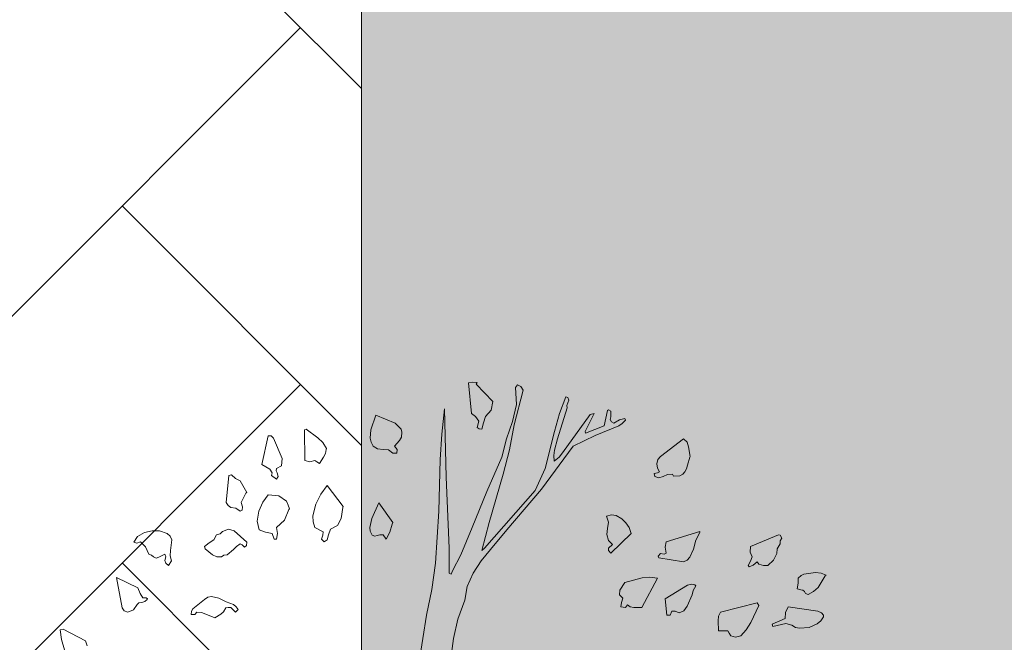
# Model space of a CAD drawing. Units: inches. Extents: x 84 to 1044, y -280 to 906.
# Tile 5 of 105: x 441 to 481, y -104 to -79. Entities that reach past the tile are written whole.
import ezdxf

# ---------------------------------------------------------------- set-up
doc = ezdxf.new("R2010")
doc.units = ezdxf.units.IN
doc.layers.add('L-HRDS', color=32, linetype='Continuous', lineweight=18)
doc.layers.add('L-PLNT', color=114, linetype='Continuous', lineweight=15)
doc.layers.add('L-PLNT-PATT', color=9, linetype='Continuous', lineweight=9, true_color=0xafd9aa)
doc.layers.add('L-PRKG-PATT', color=35, linetype='Continuous', lineweight=9, true_color=0x947764)

# ---------------------------------------------------------------- blocks, each defined once
blk = doc.blocks.new('A$C37E508DF')
for p, q in [((0.6329, 1.5111), (0.6367, 1.5175)), ((0.6367, 1.5175), (0.6423, 1.5201)), ((0.6423, 1.5201), (0.6453, 1.5158)), ((0.6453, 1.5158), (0.644, 1.4879)), ((0.6826, 1.493), (0.7096, 1.5209)), ((0.7083, 1.5239), (0.7152, 1.5244)), ((0.7096, 1.5209), (0.7083, 1.5239)), ((0.7152, 1.5244), (0.7225, 1.5231)), ((0.7225, 1.5231), (0.7174, 1.4729)), ((0.5583, 1.4948), (0.5596, 1.4995)), ((0.5596, 1.4995), (0.563, 1.5003)), ((0.563, 1.5003), (0.5737, 1.4733)), ((0.6475, 1.4545), (0.6329, 1.5111)), ((0.5596, 1.4905), (0.5583, 1.4948)), ((0.5613, 1.4862), (0.5596, 1.4905)), ((0.5608, 1.4823), (0.5613, 1.4862)), ((0.5767, 1.4317), (0.5608, 1.4823)), ((0.644, 1.4879), (0.6505, 1.46)), ((0.6852, 1.4785), (0.6826, 1.493)), ((0.7589, 1.3691), (0.7615, 1.481)), ((0.7615, 1.481), (0.7658, 1.4395)), ((0.4657, 1.4622), (0.4669, 1.4652)), ((0.4669, 1.4652), (0.4755, 1.463)), ((0.4897, 1.4772), (0.4935, 1.4789)), ((0.4897, 1.4678), (0.4897, 1.4772)), ((0.4905, 1.4635), (0.4897, 1.4678)), ((0.4935, 1.4789), (0.4952, 1.478)), ((0.4952, 1.478), (0.5004, 1.4532)), ((0.5313, 1.4437), (0.5167, 1.4729)), ((0.5167, 1.4729), (0.5231, 1.4716)), ((0.5231, 1.4716), (0.5686, 1.409)), ((0.5737, 1.4733), (0.5814, 1.4437)), ((0.6946, 1.4682), (0.6852, 1.4785)), ((0.6976, 1.4579), (0.6946, 1.4682)), ((0.7109, 1.4682), (0.7053, 1.4609)), ((0.7174, 1.4729), (0.7109, 1.4682)), ((0.8421, 1.4575), (0.8739, 1.4703)), ((0.8739, 1.4703), (0.882, 1.4463)), ((0.4708, 1.4566), (0.4657, 1.4622)), ((0.4764, 1.4532), (0.4708, 1.4566)), ((0.4755, 1.463), (0.4845, 1.4575)), ((0.5154, 1.4373), (0.4764, 1.4532)), ((0.4845, 1.4575), (0.4884, 1.4596)), ((0.4884, 1.4596), (0.4905, 1.4635)), ((0.5004, 1.4532), (0.5308, 1.4412)), ((0.6552, 1.4137), (0.6475, 1.4545)), ((0.6505, 1.46), (0.6603, 1.4317)), ((0.7002, 1.4476), (0.6976, 1.4579)), ((0.7083, 1.4502), (0.7049, 1.448)), ((0.7053, 1.4609), (0.7083, 1.4502)), ((0.8323, 1.4476), (0.8357, 1.451)), ((0.8357, 1.451), (0.8421, 1.4575)), ((0.551, 1.4197), (0.5154, 1.4373)), ((0.5308, 1.4412), (0.5313, 1.4437)), ((0.5814, 1.4437), (0.5969, 1.3833)), ((0.7049, 1.448), (0.7002, 1.4476)), ((0.7658, 1.4395), (0.7684, 1.3979)), ((0.831, 1.4424), (0.8323, 1.4476)), ((0.8318, 1.4343), (0.831, 1.4424)), ((0.8353, 1.4292), (0.8318, 1.4343)), ((0.8829, 1.433), (0.8816, 1.4262)), ((0.882, 1.4463), (0.8829, 1.433)), ((0.9605, 1.4257), (0.9686, 1.4334)), ((0.9686, 1.4334), (0.9875, 1.4476)), ((0.9875, 1.4476), (0.9905, 1.4467)), ((0.9905, 1.4467), (0.9896, 1.3966)), ((1.0269, 1.3996), (1.0411, 1.433)), ((1.0411, 1.433), (1.045, 1.4365)), ((1.045, 1.4365), (1.0497, 1.4369)), ((1.0497, 1.4369), (1.0604, 1.3901)), ((0.3598, 1.403), (0.3628, 1.4189)), ((0.3628, 1.4189), (0.3649, 1.4266)), ((0.3649, 1.4266), (0.3709, 1.4317)), ((0.3709, 1.4317), (0.4086, 1.403)), ((0.6029, 1.3494), (0.551, 1.4197)), ((0.5814, 1.4133), (0.5767, 1.4317)), ((0.6603, 1.4317), (0.668, 1.4021)), ((0.8434, 1.4197), (0.8353, 1.4292)), ((0.8391, 1.4141), (0.8434, 1.4197)), ((0.8781, 1.4197), (0.8709, 1.4154)), ((0.8816, 1.4262), (0.8781, 1.4197)), ((0.9545, 1.4159), (0.9605, 1.4257)), ((0.3602, 1.4021), (0.3598, 1.403)), ((0.364, 1.3888), (0.3602, 1.4021)), ((0.4086, 1.403), (0.4125, 1.3979)), ((0.5686, 1.409), (0.5741, 1.4021)), ((0.5741, 1.4021), (0.5823, 1.3953)), ((0.5827, 1.4043), (0.5814, 1.4133)), ((0.5823, 1.3953), (0.5827, 1.4043)), ((0.6655, 1.3743), (0.6552, 1.4137)), ((0.668, 1.4021), (0.6925, 1.3455)), ((0.8395, 1.4086), (0.8391, 1.4141)), ((0.846, 1.4086), (0.8395, 1.4086)), ((0.8528, 1.4137), (0.846, 1.4086)), ((0.8619, 1.4146), (0.8528, 1.4137)), ((0.8709, 1.4154), (0.8619, 1.4146)), ((0.9549, 1.4146), (0.9545, 1.4159)), ((0.9558, 1.4077), (0.9549, 1.4146)), ((0.9592, 1.4017), (0.9558, 1.4077)), ((0.966, 1.3914), (0.9592, 1.4017)), ((0.3657, 1.3828), (0.364, 1.3888)), ((0.4125, 1.3979), (0.4142, 1.391)), ((0.4142, 1.391), (0.4134, 1.3837)), ((0.7684, 1.3979), (0.771, 1.3134)), ((0.9703, 1.3944), (0.966, 1.3914)), ((0.9733, 1.3966), (0.9703, 1.3944)), ((0.9819, 1.3944), (0.9733, 1.3966)), ((0.9896, 1.3966), (0.9819, 1.3944)), ((1.0282, 1.3876), (1.0269, 1.3996)), ((1.0359, 1.3833), (1.0282, 1.3876)), ((1.0604, 1.3901), (1.0471, 1.3824)), ((0.3683, 1.3781), (0.3657, 1.3828)), ((0.3718, 1.3738), (0.3683, 1.3781)), ((0.3765, 1.3713), (0.3718, 1.3738)), ((0.3872, 1.3708), (0.3765, 1.3713)), ((0.3885, 1.3738), (0.3872, 1.3708)), ((0.3971, 1.3734), (0.3885, 1.3738)), ((0.4039, 1.3704), (0.3971, 1.3734)), ((0.4108, 1.3683), (0.4039, 1.3704)), ((0.4134, 1.3837), (0.4099, 1.3781)), ((0.4099, 1.3781), (0.4134, 1.376)), ((0.4176, 1.37), (0.4108, 1.3683)), ((0.4134, 1.376), (0.4189, 1.3751)), ((0.4189, 1.3751), (0.4176, 1.37)), ((0.5969, 1.3833), (0.6132, 1.3472)), ((0.6882, 1.2949), (0.6655, 1.3743)), ((0.7538, 1.2529), (0.7589, 1.3691)), ((1.0334, 1.37), (1.0351, 1.376)), ((1.0359, 1.3661), (1.0334, 1.37)), ((1.0351, 1.376), (1.0368, 1.3794)), ((1.0368, 1.3794), (1.0359, 1.3833)), ((1.0441, 1.3717), (1.0359, 1.3661)), ((1.0471, 1.3824), (1.0432, 1.3764)), ((1.0432, 1.3764), (1.0441, 1.3717)), ((1.1033, 1.367), (1.1097, 1.373)), ((1.1097, 1.373), (1.114, 1.3717)), ((1.114, 1.3717), (1.1183, 1.328)), ((0.9274, 1.3215), (0.9532, 1.3554)), ((0.9532, 1.3554), (0.9635, 1.3413)), ((1.0848, 1.3443), (1.0955, 1.3631)), ((1.0955, 1.3631), (1.1033, 1.367)), ((0.6595, 1.2829), (0.6029, 1.3494)), ((0.6132, 1.3472), (0.6959, 1.2529)), ((0.6925, 1.3455), (0.7161, 1.2868)), ((0.9635, 1.3413), (0.9721, 1.325)), ((1.0197, 1.3297), (1.0321, 1.3387)), ((1.0321, 1.3387), (1.0497, 1.3404)), ((1.0497, 1.3404), (1.0587, 1.3284)), ((1.0861, 1.343), (1.0848, 1.3443)), ((1.0938, 1.328), (1.0861, 1.343)), ((0.846, 1.2949), (0.8687, 1.3271)), ((0.8687, 1.3271), (0.8803, 1.3014)), ((0.9279, 1.3194), (0.9274, 1.3215)), ((0.9721, 1.325), (0.9768, 1.3061)), ((1.0149, 1.3172), (1.0171, 1.3232)), ((1.0171, 1.3232), (1.0197, 1.3297)), ((1.0587, 1.3284), (1.0651, 1.3134)), ((1.0917, 1.3207), (1.0938, 1.328)), ((1.0925, 1.3151), (1.0917, 1.3207)), ((1.1153, 1.3228), (1.111, 1.3194)), ((1.1183, 1.328), (1.1153, 1.3228)), ((0.4717, 1.3009), (0.4807, 1.3065)), ((0.4807, 1.3065), (0.4884, 1.3074)), ((0.4884, 1.3074), (0.4965, 1.3057)), ((0.4965, 1.3057), (0.4935, 1.2954)), ((0.771, 1.3134), (0.7761, 1.2285)), ((0.9305, 1.3018), (0.9279, 1.3194)), ((0.9768, 1.3061), (0.9763, 1.2962)), ((1.0162, 1.3164), (1.0149, 1.3172)), ((1.0231, 1.2988), (1.0162, 1.3164)), ((1.0651, 1.3134), (1.0677, 1.2975)), ((1.0955, 1.3138), (1.0925, 1.3151)), ((1.1028, 1.3185), (1.0955, 1.3138)), ((1.111, 1.3194), (1.1028, 1.3185)), ((0.4597, 1.2868), (0.4648, 1.2945)), ((0.4648, 1.2945), (0.4717, 1.3009)), ((0.4935, 1.2954), (0.4948, 1.2855)), ((0.7002, 1.2495), (0.6882, 1.2949)), ((0.8473, 1.2924), (0.846, 1.2949)), ((0.8507, 1.2795), (0.8473, 1.2924)), ((0.8803, 1.3014), (0.8833, 1.2872)), ((0.9365, 1.2902), (0.9305, 1.3018)), ((0.9476, 1.2842), (0.9365, 1.2902)), ((0.9763, 1.2962), (0.9733, 1.2868)), ((1.0359, 1.2868), (1.0231, 1.2988)), ((1.0677, 1.2975), (1.0647, 1.2829)), ((0.2101, 1.2696), (0.2127, 1.2744)), ((0.2127, 1.2744), (0.2152, 1.2752)), ((0.2152, 1.2752), (0.2611, 1.2559)), ((0.3439, 1.2804), (0.3992, 1.2636)), ((0.3439, 1.2787), (0.3439, 1.2804)), ((0.3507, 1.2662), (0.3439, 1.2787)), ((0.4562, 1.2774), (0.4597, 1.2868)), ((0.4897, 1.2452), (0.4562, 1.2774)), ((0.4961, 1.2756), (0.4935, 1.2658)), ((0.4948, 1.2855), (0.4961, 1.2756)), ((0.6865, 1.2508), (0.6595, 1.2829)), ((0.7161, 1.2868), (0.7349, 1.2422)), ((0.8567, 1.2679), (0.8507, 1.2795)), ((0.8619, 1.2752), (0.8567, 1.2679)), ((0.867, 1.2752), (0.8619, 1.2752)), ((0.8713, 1.2739), (0.867, 1.2752)), ((0.8756, 1.2726), (0.8713, 1.2739)), ((0.8799, 1.2744), (0.8756, 1.2726)), ((0.8829, 1.2808), (0.8799, 1.2744)), ((0.8833, 1.2872), (0.8829, 1.2808)), ((0.951, 1.2748), (0.9476, 1.2842)), ((0.9532, 1.2666), (0.951, 1.2748)), ((0.9733, 1.2868), (0.9596, 1.2799)), ((0.9596, 1.2799), (0.9605, 1.2744)), ((0.9605, 1.2744), (0.9626, 1.2679)), ((1.0347, 1.2769), (1.0359, 1.2868)), ((1.0359, 1.2679), (1.0347, 1.2769)), ((1.0432, 1.2774), (1.0402, 1.2679)), ((1.0544, 1.2791), (1.0432, 1.2774)), ((1.0647, 1.2829), (1.0544, 1.2791)), ((1.0848, 1.2628), (1.1054, 1.2817)), ((1.1054, 1.2817), (1.1148, 1.2842)), ((1.1148, 1.2842), (1.1247, 1.2804)), ((1.1247, 1.2804), (1.1281, 1.2765)), ((1.1281, 1.2765), (1.1341, 1.2752)), ((1.1341, 1.2752), (1.1384, 1.2666)), ((1.2075, 1.2666), (1.21, 1.2726)), ((1.21, 1.2726), (1.2147, 1.2774)), ((1.2147, 1.2774), (1.2276, 1.2817)), ((1.2276, 1.2817), (1.2392, 1.2817)), ((1.2392, 1.2817), (1.2521, 1.2787)), ((1.2521, 1.2787), (1.2632, 1.2722)), ((1.2632, 1.2722), (1.2692, 1.2628)), ((0.2127, 1.2654), (0.2101, 1.2696)), ((0.2127, 1.2602), (0.2127, 1.2654)), ((0.2174, 1.2521), (0.2127, 1.2602)), ((0.2611, 1.2559), (0.262, 1.2465)), ((0.3546, 1.2516), (0.3507, 1.2662)), ((0.3992, 1.2636), (0.4005, 1.2546)), ((0.4935, 1.2658), (0.4867, 1.2589)), ((0.4867, 1.2589), (0.4935, 1.2529)), ((0.9583, 1.2636), (0.9532, 1.2666)), ((0.9626, 1.2679), (0.9583, 1.2636)), ((1.0402, 1.2679), (1.0359, 1.2679)), ((1.0852, 1.2576), (1.0848, 1.2628)), ((1.0883, 1.2546), (1.0852, 1.2576)), ((1.0921, 1.2585), (1.0883, 1.2546)), ((1.0955, 1.2602), (1.0921, 1.2585)), ((1.1015, 1.2559), (1.0955, 1.2602)), ((1.1063, 1.2508), (1.1015, 1.2559)), ((1.1384, 1.2666), (1.1461, 1.2619)), ((1.1461, 1.2619), (1.1539, 1.2559)), ((1.1539, 1.2559), (1.1526, 1.2521)), ((1.2096, 1.2491), (1.2075, 1.2666)), ((1.2585, 1.2636), (1.2503, 1.2551)), ((1.2645, 1.2615), (1.2585, 1.2636)), ((1.2692, 1.2628), (1.2645, 1.2615)), ((0.2182, 1.2443), (0.2174, 1.2521)), ((0.2234, 1.2336), (0.2182, 1.2443)), ((0.262, 1.2465), (0.2586, 1.2388)), ((0.3602, 1.2383), (0.3546, 1.2516)), ((0.4005, 1.2546), (0.3992, 1.2452)), ((0.3992, 1.2452), (0.4026, 1.2431)), ((0.4026, 1.2431), (0.4086, 1.2443)), ((0.4086, 1.2443), (0.4121, 1.2401)), ((0.4121, 1.2401), (0.4112, 1.2375)), ((0.4931, 1.2491), (0.4897, 1.2452)), ((0.4935, 1.2529), (0.4931, 1.2491)), ((0.7015, 1.2323), (0.6865, 1.2508)), ((0.6959, 1.2529), (0.7002, 1.2495)), ((0.7349, 1.2422), (0.7482, 1.216)), ((0.7538, 1.2122), (0.7538, 1.2529)), ((1.117, 1.2422), (1.1063, 1.2508)), ((1.1221, 1.2418), (1.117, 1.2422)), ((1.126, 1.2388), (1.1221, 1.2418)), ((1.141, 1.2422), (1.1337, 1.2388)), ((1.1526, 1.2521), (1.141, 1.2422)), ((1.2079, 1.2323), (1.21, 1.2409)), ((1.21, 1.2409), (1.2096, 1.2491)), ((1.2186, 1.2431), (1.2173, 1.2392)), ((1.2285, 1.2383), (1.2186, 1.2431)), ((1.2405, 1.2418), (1.2371, 1.2388)), ((1.2448, 1.2431), (1.2405, 1.2418)), ((1.2503, 1.2551), (1.2448, 1.2431)), ((0.2328, 1.2251), (0.2234, 1.2336)), ((0.2401, 1.2251), (0.2328, 1.2251)), ((0.2474, 1.2268), (0.2401, 1.2251)), ((0.2504, 1.2306), (0.2474, 1.2268)), ((0.2568, 1.2255), (0.2504, 1.2306)), ((0.2633, 1.2229), (0.2568, 1.2255)), ((0.2586, 1.2388), (0.2611, 1.2319)), ((0.2611, 1.2319), (0.265, 1.2251)), ((0.265, 1.2251), (0.2633, 1.2229)), ((0.3649, 1.2336), (0.3602, 1.2383)), ((0.3709, 1.2306), (0.3649, 1.2336)), ((0.4112, 1.2375), (0.3709, 1.2306)), ((0.7148, 1.2126), (0.7015, 1.2323)), ((0.7761, 1.2285), (0.7821, 1.1856)), ((1.1337, 1.2388), (1.126, 1.2388)), ((1.2126, 1.2251), (1.2079, 1.2323)), ((1.2169, 1.2285), (1.2126, 1.2251)), ((1.2186, 1.2332), (1.2169, 1.2285)), ((1.2173, 1.2392), (1.2186, 1.2332)), ((1.2328, 1.2366), (1.2285, 1.2383)), ((1.2371, 1.2388), (1.2328, 1.2366)), ((0.1376, 1.2092), (0.1458, 1.2126)), ((0.1389, 1.2079), (0.1376, 1.2092)), ((0.1505, 1.189), (0.1389, 1.2079)), ((0.1458, 1.2126), (0.1548, 1.2135)), ((0.1548, 1.2135), (0.1741, 1.2109)), ((0.1741, 1.2109), (0.1784, 1.2083)), ((0.1784, 1.2083), (0.1831, 1.204)), ((0.7246, 1.1908), (0.7148, 1.2126)), ((0.7482, 1.216), (0.7508, 1.2109)), ((0.7508, 1.2109), (0.7538, 1.2122)), ((0.1831, 1.204), (0.1831, 1.1959)), ((0.1831, 1.1959), (0.1848, 1.1865)), ((0.3507, 1.1916), (0.352, 1.1933)), ((0.355, 1.1839), (0.3507, 1.1916)), ((0.352, 1.1933), (0.3576, 1.1942)), ((0.3576, 1.1942), (0.364, 1.1929)), ((0.364, 1.1929), (0.4005, 1.1702)), ((0.4134, 1.204), (0.4258, 1.2058)), ((0.4391, 1.156), (0.4134, 1.204)), ((0.4258, 1.2058), (0.4382, 1.2045)), ((0.4382, 1.2045), (0.4669, 1.1972)), ((0.4669, 1.1972), (0.4747, 1.1843)), ((1.2628, 1.1882), (1.2975, 1.2053)), ((1.2975, 1.2053), (1.2885, 1.1556)), ((0.1582, 1.1822), (0.1505, 1.189)), ((0.1668, 1.1775), (0.1582, 1.1822)), ((0.1711, 1.1792), (0.1668, 1.1775)), ((0.1728, 1.1826), (0.1711, 1.1792)), ((0.1758, 1.1847), (0.1728, 1.1826)), ((0.1788, 1.1852), (0.1758, 1.1847)), ((0.1848, 1.1865), (0.1788, 1.1852)), ((0.3563, 1.177), (0.355, 1.1839)), ((0.3645, 1.1586), (0.3563, 1.177)), ((0.4751, 1.177), (0.47, 1.1714)), ((0.4747, 1.1843), (0.4751, 1.177)), ((0.7281, 1.168), (0.7246, 1.1908)), ((0.7821, 1.1856), (0.7911, 1.1436)), ((1.2546, 1.1719), (1.2589, 1.1792)), ((1.2589, 1.1792), (1.2628, 1.1882)), ((0.2478, 1.1594), (0.2504, 1.1637)), ((0.2607, 1.1316), (0.2478, 1.1594)), ((0.2504, 1.1637), (0.3104, 1.1487)), ((0.4005, 1.1702), (0.3979, 1.1436)), ((0.4622, 1.1607), (0.458, 1.1573)), ((0.4657, 1.156), (0.4622, 1.1607)), ((0.47, 1.1714), (0.4721, 1.1646)), ((0.4721, 1.1646), (0.473, 1.1573)), ((0.7396, 1.1371), (0.7281, 1.168)), ((1.102, 1.1573), (1.1063, 1.1612)), ((1.1063, 1.1612), (1.1187, 1.1655)), ((1.1187, 1.1655), (1.1307, 1.1714)), ((1.1307, 1.1714), (1.1423, 1.1744)), ((1.1423, 1.1744), (1.1483, 1.1732)), ((1.1483, 1.1732), (1.1539, 1.1693)), ((1.1539, 1.1693), (1.1727, 1.1543)), ((1.2469, 1.1702), (1.2495, 1.1723)), ((1.2478, 1.1693), (1.2469, 1.1702)), ((1.2516, 1.1659), (1.2478, 1.1693)), ((1.2495, 1.1723), (1.2546, 1.1719)), ((1.2563, 1.1646), (1.2516, 1.1659)), ((1.2611, 1.1637), (1.2563, 1.1646)), ((1.2641, 1.1612), (1.2611, 1.1637)), ((1.2701, 1.1522), (1.2641, 1.1612)), ((0.1419, 1.1436), (0.1449, 1.1474)), ((0.1419, 1.141), (0.1419, 1.1436)), ((0.1449, 1.1474), (0.1509, 1.1504)), ((0.1509, 1.1504), (0.1994, 1.1573)), ((0.1994, 1.1573), (0.2041, 1.1479)), ((0.2041, 1.1479), (0.2045, 1.138)), ((0.3104, 1.1487), (0.3134, 1.1423)), ((0.37, 1.1509), (0.3645, 1.1586)), ((0.3778, 1.1474), (0.37, 1.1509)), ((0.3842, 1.15), (0.3778, 1.1474)), ((0.3898, 1.15), (0.3842, 1.15)), ((0.3923, 1.1436), (0.3898, 1.15)), ((0.3979, 1.1436), (0.3923, 1.1436)), ((0.4519, 1.1564), (0.4391, 1.156)), ((0.458, 1.1573), (0.4519, 1.1564)), ((0.473, 1.1573), (0.4657, 1.156)), ((0.7911, 1.1436), (0.8027, 1.0677)), ((1.099, 1.153), (1.102, 1.1573)), ((1.1033, 1.1487), (1.099, 1.153)), ((1.111, 1.156), (1.1033, 1.1487)), ((1.1153, 1.1564), (1.111, 1.156)), ((1.1191, 1.1556), (1.1153, 1.1564)), ((1.1226, 1.1492), (1.1191, 1.1556)), ((1.1273, 1.1453), (1.1226, 1.1492)), ((1.1367, 1.1393), (1.1273, 1.1453)), ((1.1517, 1.1453), (1.1367, 1.1393)), ((1.1586, 1.1483), (1.1517, 1.1453)), ((1.1663, 1.1487), (1.1586, 1.1483)), ((1.1697, 1.1449), (1.1663, 1.1487)), ((1.1757, 1.1449), (1.1697, 1.1449)), ((1.1727, 1.1543), (1.1749, 1.1504)), ((1.1749, 1.1504), (1.1757, 1.1449)), ((1.2791, 1.1487), (1.2701, 1.1522)), ((1.2851, 1.1509), (1.2791, 1.1487)), ((1.2885, 1.1556), (1.2851, 1.1509)), ((0.1462, 1.1342), (0.1419, 1.141)), ((0.1522, 1.1294), (0.1462, 1.1342)), ((0.1655, 1.1234), (0.1522, 1.1294)), ((0.1938, 1.1273), (0.1878, 1.1234)), ((0.2032, 1.1303), (0.1938, 1.1273)), ((0.2247, 1.1251), (0.2032, 1.1303)), ((0.2045, 1.138), (0.226, 1.129)), ((0.226, 1.129), (0.2247, 1.1251)), ((0.268, 1.1196), (0.2607, 1.1316)), ((0.3134, 1.1423), (0.3139, 1.1346)), ((0.3139, 1.1346), (0.3134, 1.1183)), ((0.7469, 1.1054), (0.7396, 1.1371)), ((0.181, 1.1226), (0.1655, 1.1234)), ((0.1878, 1.1234), (0.181, 1.1226)), ((0.277, 1.1101), (0.268, 1.1196)), ((0.2959, 1.1144), (0.2933, 1.1101)), ((0.2984, 1.1179), (0.2959, 1.1144)), ((0.3066, 1.1179), (0.2984, 1.1179)), ((0.3134, 1.1183), (0.3066, 1.1179)), ((1.3485, 1.102), (1.385, 1.1209)), ((1.385, 1.1209), (1.3897, 1.1196)), ((1.3897, 1.1196), (1.3875, 1.1037)), ((0.2856, 1.108), (0.277, 1.1101)), ((0.2933, 1.1101), (0.2856, 1.108)), ((0.7512, 1.0728), (0.7469, 1.1054)), ((1.3455, 1.0934), (1.3485, 1.102)), ((1.3875, 1.1037), (1.3828, 1.087))]:
    blk.add_line(p, q)

msp = doc.modelspace()

# ---------------------------------------------------------------- hatches: boundary and pattern name
at = {"layer": 'L-PLNT-PATT', "transparency": 33554597}
h = msp.add_hatch(color=256, dxfattribs=at)
h.dxf.hatch_style = 1
h.paths.add_polyline_path([(504.574, -40.88), (455.074, -40.88), (455.074, -112.88), (504.574, -112.88)])
at = {"layer": 'L-PRKG-PATT', "transparency": 33554567}
h = msp.add_hatch(dxfattribs=at)
h.set_pattern_fill('AR-HBONE', color=256, scale=0.1)
h.paths.add_polyline_path([(455.074, 31.12), (455.074, 91.12), (455.074, 151.12), (413.127, 151.12), (341.127, 151.12), (290.179, 151.12), (227.179, 151.12), (227.179, 127.12), (143.179, 127.12), (143.179, -112.88), (143.179, -117.88), (455.074, -117.88)])

# ---------------------------------------------------------------- linework, layer by layer
at = {"layer": 'L-HRDS'}
msp.add_line((455.074, 31.12), (455.074, -121.88), dxfattribs=at)

# ---------------------------------------------------------------- block references
at = {"layer": 'L-PLNT', "xscale": -24.64361536662419, "yscale": 24.64361536662419, "zscale": 24.64361536662419}
msp.add_blockref('A$C37E508DF', (477.187, -130.86), dxfattribs=at)

doc.saveas('drawing.dxf')
